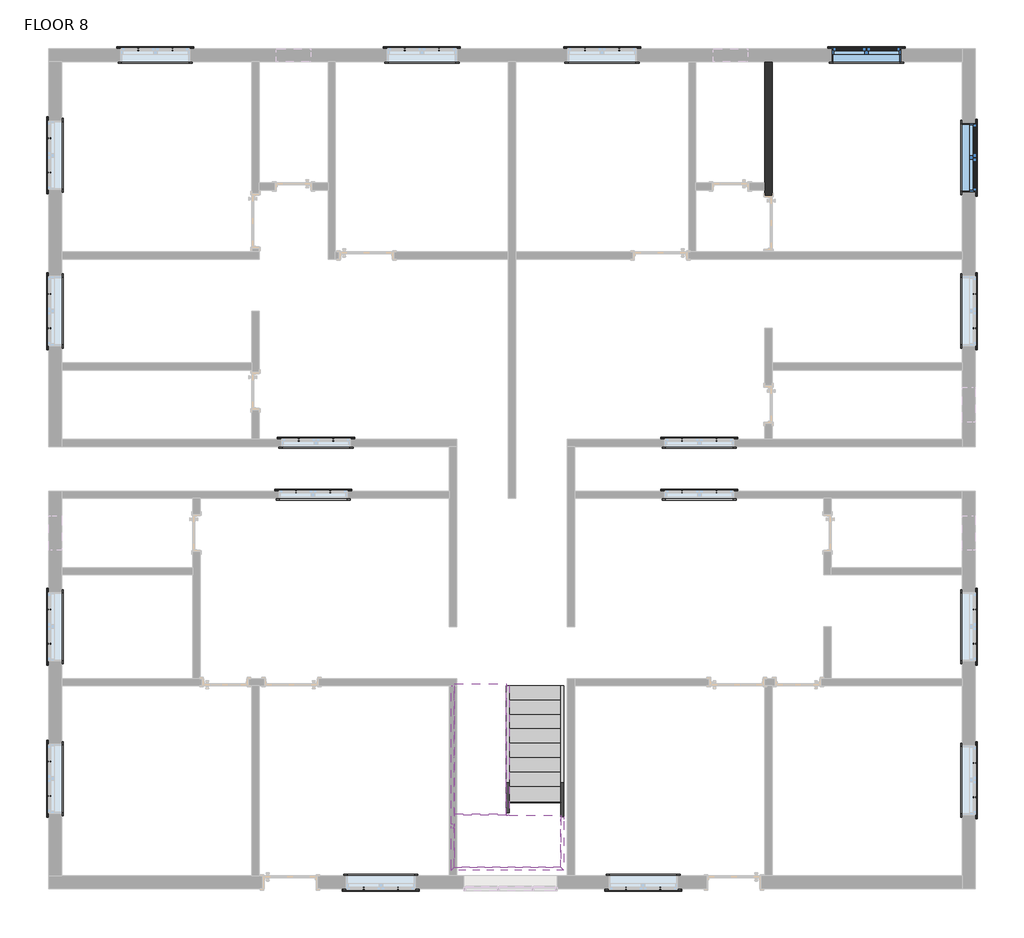
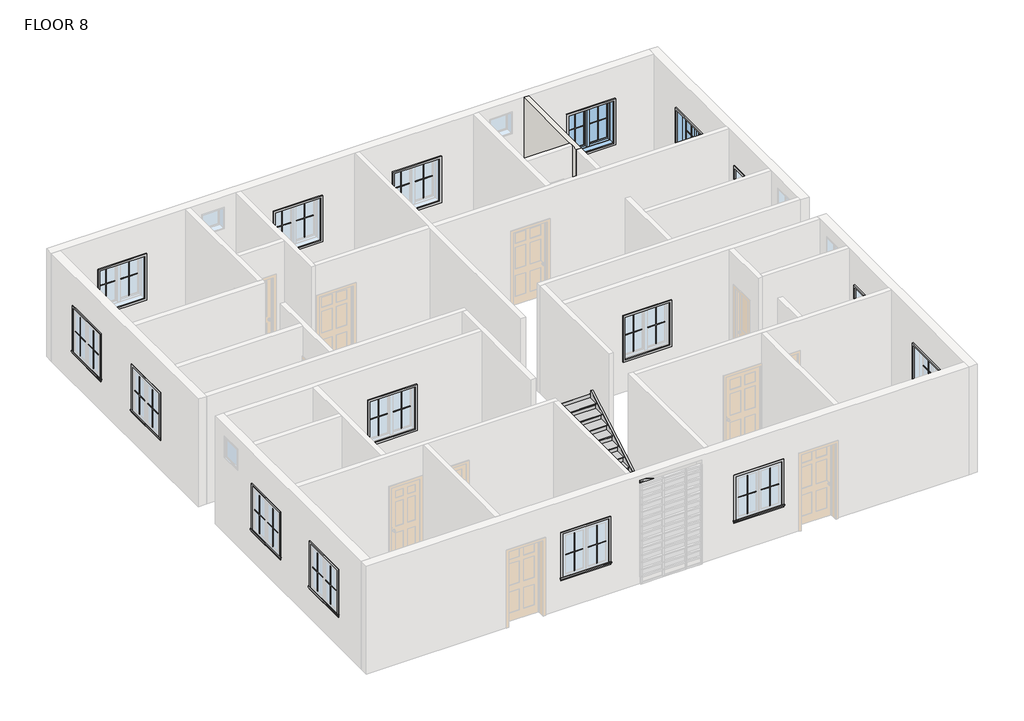
# One storey, part 4 of 4: 72 proxies, 7 members, 2 stair flights, 2 windows, 1 slab, 1 wall.
"""IFC4 building model written with IfcOpenShell, lengths in millimetres."""

from ifc_helpers import new_model, si_unit, frame, origin, place, context, project, spatial, polyline, outline, extrude, faceted_brep, transform, mapped, element, save
from components import muntin_pattern_2x2_muntin_pattern_2x2_4dfeb3f3, muntin_pattern_2x2_muntin_pattern_2x2_e852a7e4, trim_window_exterior_flat_with_sill_7cfdd449, trim_window_interior_flat_picture_frame_f1e0b15b, non_monolithic_landing_a6268fe4, stair_flight_98d8f9c6, stair_flight_dd50f657, window_9200f5ac

model = new_model("IFC4")

# Units and contexts
model_context = context("Model", 3, world=origin())
ifc_project = project(units=[si_unit("LENGTHUNIT", "METRE", prefix="MILLI")], contexts=[model_context])

# Site, building, storey
site = spatial("IfcSite", under=ifc_project)
building = spatial("IfcBuilding", under=site)
storey = spatial("IfcBuildingStorey", under=building, Name="FLOOR 8", Elevation=12744.7725604)

# Proxies
placement = place(None, origin())
muntin_pattern_2x2_muntin_pattern_2x2_shape = muntin_pattern_2x2_muntin_pattern_2x2_4dfeb3f3(model_context)
element("IfcBuildingElementProxy", 1, Name="Muntin Pattern_2x2 : Muntin Pattern_2x2", ObjectType="Muntin Pattern_2x2 : Muntin Pattern_2x2", at=placement, inside=storey, context=model_context, shape_type="MappedRepresentation", body=[
    mapped(muntin_pattern_2x2_muntin_pattern_2x2_shape, transform((-12420.8887331, 2059.7281164, 13729.0225604), x_axis=(0.0, 1.0, 0.0), y_axis=(-1.0, 0.0, 0.0), z_axis=(0.0, 0.0, 1.0))),
])
element("IfcBuildingElementProxy", 2, Name="Muntin Pattern_2x2 : Muntin Pattern_2x2", ObjectType="Muntin Pattern_2x2 : Muntin Pattern_2x2", at=placement, inside=storey, context=model_context, shape_type="MappedRepresentation", body=[
    mapped(muntin_pattern_2x2_muntin_pattern_2x2_shape, transform((-12420.8887331, 4803.7218664, 13729.0225604), x_axis=(0.0, 1.0, 0.0), y_axis=(-1.0, 0.0, 0.0), z_axis=(0.0, 0.0, 1.0))),
])
element("IfcBuildingElementProxy", 3, Name="Muntin Pattern_2x2 : Muntin Pattern_2x2", ObjectType="Muntin Pattern_2x2 : Muntin Pattern_2x2", at=placement, inside=storey, context=model_context, shape_type="MappedRepresentation", body=[
    mapped(muntin_pattern_2x2_muntin_pattern_2x2_shape, transform((-10854.0262331, 6977.8031164, 13729.0225604), x_axis=(1.0, 0.0, 0.0), y_axis=(0.0, 1.0, 0.0), z_axis=(0.0, 0.0, 1.0))),
])
element("IfcBuildingElementProxy", 4, Name="Muntin Pattern_2x2 : Muntin Pattern_2x2", ObjectType="Muntin Pattern_2x2 : Muntin Pattern_2x2", at=placement, inside=storey, context=model_context, shape_type="MappedRepresentation", body=[
    mapped(muntin_pattern_2x2_muntin_pattern_2x2_shape, transform((-6155.0262331, 6977.8031164, 13729.0225604), x_axis=(1.0, 0.0, 0.0), y_axis=(0.0, 1.0, 0.0), z_axis=(0.0, 0.0, 1.0))),
])
element("IfcBuildingElementProxy", 5, Name="Muntin Pattern_2x2 : Muntin Pattern_2x2", ObjectType="Muntin Pattern_2x2 : Muntin Pattern_2x2", at=placement, inside=storey, context=model_context, shape_type="MappedRepresentation", body=[
    mapped(muntin_pattern_2x2_muntin_pattern_2x2_shape, transform((-2980.0262331, 6977.8031164, 13729.0225604), x_axis=(1.0, 0.0, 0.0), y_axis=(0.0, 1.0, 0.0), z_axis=(0.0, 0.0, 1.0))),
])
element("IfcBuildingElementProxy", 6, Name="Muntin Pattern_2x2 : Muntin Pattern_2x2", ObjectType="Muntin Pattern_2x2 : Muntin Pattern_2x2", at=placement, inside=storey, context=model_context, shape_type="MappedRepresentation", body=[
    mapped(muntin_pattern_2x2_muntin_pattern_2x2_shape, transform((1680.8737669, 6977.8031164, 13729.0225604), x_axis=(1.0, 0.0, 0.0), y_axis=(0.0, 1.0, 0.0), z_axis=(0.0, 0.0, 1.0))),
])
element("IfcBuildingElementProxy", 7, Name="Muntin Pattern_2x2 : Muntin Pattern_2x2", ObjectType="Muntin Pattern_2x2 : Muntin Pattern_2x2", at=placement, inside=storey, context=model_context, shape_type="MappedRepresentation", body=[
    mapped(muntin_pattern_2x2_muntin_pattern_2x2_shape, transform((3892.2612669, 5371.2531164, 13729.0225604), x_axis=(0.0, -1.0, 0.0), y_axis=(1.0, 0.0, 0.0), z_axis=(0.0, 0.0, 1.0))),
])
element("IfcBuildingElementProxy", 8, Name="Muntin Pattern_2x2 : Muntin Pattern_2x2", ObjectType="Muntin Pattern_2x2 : Muntin Pattern_2x2", at=placement, inside=storey, context=model_context, shape_type="MappedRepresentation", body=[
    mapped(muntin_pattern_2x2_muntin_pattern_2x2_shape, transform((3892.2612669, 2666.1531164, 13729.0225604), x_axis=(0.0, -1.0, 0.0), y_axis=(1.0, 0.0, 0.0), z_axis=(0.0, 0.0, 1.0))),
])
element("IfcBuildingElementProxy", 9, Name="Muntin Pattern_2x2 : Muntin Pattern_2x2", ObjectType="Muntin Pattern_2x2 : Muntin Pattern_2x2", at=placement, inside=storey, context=model_context, shape_type="MappedRepresentation", body=[
    mapped(muntin_pattern_2x2_muntin_pattern_2x2_shape, transform((3892.2612669, -2896.4468836, 13729.0225604), x_axis=(0.0, -1.0, 0.0), y_axis=(1.0, 0.0, 0.0), z_axis=(0.0, 0.0, 1.0))),
])
element("IfcBuildingElementProxy", 10, Name="Muntin Pattern_2x2 : Muntin Pattern_2x2", ObjectType="Muntin Pattern_2x2 : Muntin Pattern_2x2", at=placement, inside=storey, context=model_context, shape_type="MappedRepresentation", body=[
    mapped(muntin_pattern_2x2_muntin_pattern_2x2_shape, transform((3892.2612669, -5601.5468836, 13729.0225604), x_axis=(0.0, -1.0, 0.0), y_axis=(1.0, 0.0, 0.0), z_axis=(0.0, 0.0, 1.0))),
])
element("IfcBuildingElementProxy", 11, Name="Muntin Pattern_2x2 : Muntin Pattern_2x2", ObjectType="Muntin Pattern_2x2 : Muntin Pattern_2x2", at=placement, inside=storey, context=model_context, shape_type="MappedRepresentation", body=[
    mapped(muntin_pattern_2x2_muntin_pattern_2x2_shape, transform((-1649.7012331, -7812.9343836, 13729.0225604), x_axis=(-1.0, 0.0, 0.0), y_axis=(0.0, -1.0, 0.0), z_axis=(0.0, 0.0, 1.0))),
])
element("IfcBuildingElementProxy", 12, Name="Muntin Pattern_2x2 : Muntin Pattern_2x2", ObjectType="Muntin Pattern_2x2 : Muntin Pattern_2x2", at=placement, inside=storey, context=model_context, shape_type="MappedRepresentation", body=[
    mapped(muntin_pattern_2x2_muntin_pattern_2x2_shape, transform((-6272.5012331, -7812.9343836, 13729.0225604), x_axis=(-1.0, 0.0, 0.0), y_axis=(0.0, -1.0, 0.0), z_axis=(0.0, 0.0, 1.0))),
])
element("IfcBuildingElementProxy", 13, Name="Muntin Pattern_2x2 : Muntin Pattern_2x2", ObjectType="Muntin Pattern_2x2 : Muntin Pattern_2x2", at=placement, inside=storey, context=model_context, shape_type="MappedRepresentation", body=[
    mapped(muntin_pattern_2x2_muntin_pattern_2x2_shape, transform((-12420.8887331, -6182.5718836, 13729.0225604), x_axis=(0.0, 1.0, 0.0), y_axis=(-1.0, 0.0, 0.0), z_axis=(0.0, 0.0, 1.0))),
])
element("IfcBuildingElementProxy", 14, Name="Muntin Pattern_2x2 : Muntin Pattern_2x2", ObjectType="Muntin Pattern_2x2 : Muntin Pattern_2x2", at=placement, inside=storey, context=model_context, shape_type="MappedRepresentation", body=[
    mapped(muntin_pattern_2x2_muntin_pattern_2x2_shape, transform((-12420.8887331, -3502.8718836, 13729.0225604), x_axis=(0.0, 1.0, 0.0), y_axis=(-1.0, 0.0, 0.0), z_axis=(0.0, 0.0, 1.0))),
])
element("IfcBuildingElementProxy", 15, Name="Muntin Pattern_2x2 : Muntin Pattern_2x2", ObjectType="Muntin Pattern_2x2 : Muntin Pattern_2x2", at=placement, inside=storey, context=model_context, shape_type="MappedRepresentation", body=[
    mapped(muntin_pattern_2x2_muntin_pattern_2x2_shape, transform((-8072.7262331, -821.5843836, 13729.0225604), x_axis=(1.0, 0.0, 0.0), y_axis=(0.0, 1.0, 0.0), z_axis=(0.0, 0.0, 1.0))),
])
element("IfcBuildingElementProxy", 16, Name="Muntin Pattern_2x2 : Muntin Pattern_2x2", ObjectType="Muntin Pattern_2x2 : Muntin Pattern_2x2", at=placement, inside=storey, context=model_context, shape_type="MappedRepresentation", body=[
    mapped(muntin_pattern_2x2_muntin_pattern_2x2_shape, transform((-8021.9262331, 92.8156164, 13729.0225604), x_axis=(1.0, 0.0, 0.0), y_axis=(0.0, 1.0, 0.0), z_axis=(0.0, 0.0, 1.0))),
])
element("IfcBuildingElementProxy", 17, Name="Muntin Pattern_2x2 : Muntin Pattern_2x2", ObjectType="Muntin Pattern_2x2 : Muntin Pattern_2x2", at=placement, inside=storey, context=model_context, shape_type="MappedRepresentation", body=[
    mapped(muntin_pattern_2x2_muntin_pattern_2x2_shape, transform((-1265.5262331, -821.5843836, 13729.0225604), x_axis=(1.0, 0.0, 0.0), y_axis=(0.0, 1.0, 0.0), z_axis=(0.0, 0.0, 1.0))),
])
element("IfcBuildingElementProxy", 18, Name="Muntin Pattern_2x2 : Muntin Pattern_2x2", ObjectType="Muntin Pattern_2x2 : Muntin Pattern_2x2", at=placement, inside=storey, context=model_context, shape_type="MappedRepresentation", body=[
    mapped(muntin_pattern_2x2_muntin_pattern_2x2_shape, transform((-1265.5262331, 92.8156164, 13729.0225604), x_axis=(1.0, 0.0, 0.0), y_axis=(0.0, 1.0, 0.0), z_axis=(0.0, 0.0, 1.0))),
])
muntin_pattern_2x2_muntin_pattern_2x2_2_shape = muntin_pattern_2x2_muntin_pattern_2x2_e852a7e4(model_context)
element("IfcBuildingElementProxy", 19, Name="Muntin Pattern_2x2 : Muntin Pattern_2x2", ObjectType="Muntin Pattern_2x2 : Muntin Pattern_2x2", at=placement, inside=storey, context=model_context, shape_type="MappedRepresentation", body=[
    mapped(muntin_pattern_2x2_muntin_pattern_2x2_2_shape, transform((-12420.8887331, 2666.1531164, 13729.0225604), x_axis=(0.0, -1.0, 0.0), y_axis=(1.0, 0.0, 0.0), z_axis=(0.0, 0.0, 1.0))),
])
element("IfcBuildingElementProxy", 20, Name="Muntin Pattern_2x2 : Muntin Pattern_2x2", ObjectType="Muntin Pattern_2x2 : Muntin Pattern_2x2", at=placement, inside=storey, context=model_context, shape_type="MappedRepresentation", body=[
    mapped(muntin_pattern_2x2_muntin_pattern_2x2_2_shape, transform((-12420.8887331, 5410.1468664, 13729.0225604), x_axis=(0.0, -1.0, 0.0), y_axis=(1.0, 0.0, 0.0), z_axis=(0.0, 0.0, 1.0))),
])
element("IfcBuildingElementProxy", 21, Name="Muntin Pattern_2x2 : Muntin Pattern_2x2", ObjectType="Muntin Pattern_2x2 : Muntin Pattern_2x2", at=placement, inside=storey, context=model_context, shape_type="MappedRepresentation", body=[
    mapped(muntin_pattern_2x2_muntin_pattern_2x2_2_shape, transform((-10247.6012331, 6977.8031164, 13729.0225604), x_axis=(-1.0, 0.0, 0.0), y_axis=(0.0, -1.0, 0.0), z_axis=(0.0, 0.0, 1.0))),
])
element("IfcBuildingElementProxy", 22, Name="Muntin Pattern_2x2 : Muntin Pattern_2x2", ObjectType="Muntin Pattern_2x2 : Muntin Pattern_2x2", at=placement, inside=storey, context=model_context, shape_type="MappedRepresentation", body=[
    mapped(muntin_pattern_2x2_muntin_pattern_2x2_2_shape, transform((-5548.6012331, 6977.8031164, 13729.0225604), x_axis=(-1.0, 0.0, 0.0), y_axis=(0.0, -1.0, 0.0), z_axis=(0.0, 0.0, 1.0))),
])
element("IfcBuildingElementProxy", 23, Name="Muntin Pattern_2x2 : Muntin Pattern_2x2", ObjectType="Muntin Pattern_2x2 : Muntin Pattern_2x2", at=placement, inside=storey, context=model_context, shape_type="MappedRepresentation", body=[
    mapped(muntin_pattern_2x2_muntin_pattern_2x2_2_shape, transform((-2373.6012331, 6977.8031164, 13729.0225604), x_axis=(-1.0, 0.0, 0.0), y_axis=(0.0, -1.0, 0.0), z_axis=(0.0, 0.0, 1.0))),
])
element("IfcBuildingElementProxy", 24, Name="Muntin Pattern_2x2 : Muntin Pattern_2x2", ObjectType="Muntin Pattern_2x2 : Muntin Pattern_2x2", at=placement, inside=storey, context=model_context, shape_type="MappedRepresentation", body=[
    mapped(muntin_pattern_2x2_muntin_pattern_2x2_2_shape, transform((2287.2987669, 6977.8031164, 13729.0225604), x_axis=(-1.0, 0.0, 0.0), y_axis=(0.0, -1.0, 0.0), z_axis=(0.0, 0.0, 1.0))),
])
element("IfcBuildingElementProxy", 25, Name="Muntin Pattern_2x2 : Muntin Pattern_2x2", ObjectType="Muntin Pattern_2x2 : Muntin Pattern_2x2", at=placement, inside=storey, context=model_context, shape_type="MappedRepresentation", body=[
    mapped(muntin_pattern_2x2_muntin_pattern_2x2_2_shape, transform((3892.2612669, 4764.8281164, 13729.0225604), x_axis=(0.0, 1.0, 0.0), y_axis=(-1.0, 0.0, 0.0), z_axis=(0.0, 0.0, 1.0))),
])
element("IfcBuildingElementProxy", 26, Name="Muntin Pattern_2x2 : Muntin Pattern_2x2", ObjectType="Muntin Pattern_2x2 : Muntin Pattern_2x2", at=placement, inside=storey, context=model_context, shape_type="MappedRepresentation", body=[
    mapped(muntin_pattern_2x2_muntin_pattern_2x2_2_shape, transform((3892.2612669, 2059.7281164, 13729.0225604), x_axis=(0.0, 1.0, 0.0), y_axis=(-1.0, 0.0, 0.0), z_axis=(0.0, 0.0, 1.0))),
])
element("IfcBuildingElementProxy", 27, Name="Muntin Pattern_2x2 : Muntin Pattern_2x2", ObjectType="Muntin Pattern_2x2 : Muntin Pattern_2x2", at=placement, inside=storey, context=model_context, shape_type="MappedRepresentation", body=[
    mapped(muntin_pattern_2x2_muntin_pattern_2x2_2_shape, transform((3892.2612669, -3502.8718836, 13729.0225604), x_axis=(0.0, 1.0, 0.0), y_axis=(-1.0, 0.0, 0.0), z_axis=(0.0, 0.0, 1.0))),
])
element("IfcBuildingElementProxy", 28, Name="Muntin Pattern_2x2 : Muntin Pattern_2x2", ObjectType="Muntin Pattern_2x2 : Muntin Pattern_2x2", at=placement, inside=storey, context=model_context, shape_type="MappedRepresentation", body=[
    mapped(muntin_pattern_2x2_muntin_pattern_2x2_2_shape, transform((3892.2612669, -6207.9718836, 13729.0225604), x_axis=(0.0, 1.0, 0.0), y_axis=(-1.0, 0.0, 0.0), z_axis=(0.0, 0.0, 1.0))),
])
element("IfcBuildingElementProxy", 29, Name="Muntin Pattern_2x2 : Muntin Pattern_2x2", ObjectType="Muntin Pattern_2x2 : Muntin Pattern_2x2", at=placement, inside=storey, context=model_context, shape_type="MappedRepresentation", body=[
    mapped(muntin_pattern_2x2_muntin_pattern_2x2_2_shape, transform((-2256.1262331, -7812.9343836, 13729.0225604), x_axis=(1.0, 0.0, 0.0), y_axis=(0.0, 1.0, 0.0), z_axis=(0.0, 0.0, 1.0))),
])
element("IfcBuildingElementProxy", 30, Name="Muntin Pattern_2x2 : Muntin Pattern_2x2", ObjectType="Muntin Pattern_2x2 : Muntin Pattern_2x2", at=placement, inside=storey, context=model_context, shape_type="MappedRepresentation", body=[
    mapped(muntin_pattern_2x2_muntin_pattern_2x2_2_shape, transform((-6878.9262331, -7812.9343836, 13729.0225604), x_axis=(1.0, 0.0, 0.0), y_axis=(0.0, 1.0, 0.0), z_axis=(0.0, 0.0, 1.0))),
])
element("IfcBuildingElementProxy", 31, Name="Muntin Pattern_2x2 : Muntin Pattern_2x2", ObjectType="Muntin Pattern_2x2 : Muntin Pattern_2x2", at=placement, inside=storey, context=model_context, shape_type="MappedRepresentation", body=[
    mapped(muntin_pattern_2x2_muntin_pattern_2x2_2_shape, transform((-12420.8887331, -5576.1468836, 13729.0225604), x_axis=(0.0, -1.0, 0.0), y_axis=(1.0, 0.0, 0.0), z_axis=(0.0, 0.0, 1.0))),
])
element("IfcBuildingElementProxy", 32, Name="Muntin Pattern_2x2 : Muntin Pattern_2x2", ObjectType="Muntin Pattern_2x2 : Muntin Pattern_2x2", at=placement, inside=storey, context=model_context, shape_type="MappedRepresentation", body=[
    mapped(muntin_pattern_2x2_muntin_pattern_2x2_2_shape, transform((-12420.8887331, -2896.4468836, 13729.0225604), x_axis=(0.0, -1.0, 0.0), y_axis=(1.0, 0.0, 0.0), z_axis=(0.0, 0.0, 1.0))),
])
element("IfcBuildingElementProxy", 33, Name="Muntin Pattern_2x2 : Muntin Pattern_2x2", ObjectType="Muntin Pattern_2x2 : Muntin Pattern_2x2", at=placement, inside=storey, context=model_context, shape_type="MappedRepresentation", body=[
    mapped(muntin_pattern_2x2_muntin_pattern_2x2_2_shape, transform((-7466.3012331, -821.5843836, 13729.0225604), x_axis=(-1.0, 0.0, 0.0), y_axis=(0.0, -1.0, 0.0), z_axis=(0.0, 0.0, 1.0))),
])
element("IfcBuildingElementProxy", 34, Name="Muntin Pattern_2x2 : Muntin Pattern_2x2", ObjectType="Muntin Pattern_2x2 : Muntin Pattern_2x2", at=placement, inside=storey, context=model_context, shape_type="MappedRepresentation", body=[
    mapped(muntin_pattern_2x2_muntin_pattern_2x2_2_shape, transform((-7415.5012331, 92.8156164, 13729.0225604), x_axis=(-1.0, 0.0, 0.0), y_axis=(0.0, -1.0, 0.0), z_axis=(0.0, 0.0, 1.0))),
])
element("IfcBuildingElementProxy", 35, Name="Muntin Pattern_2x2 : Muntin Pattern_2x2", ObjectType="Muntin Pattern_2x2 : Muntin Pattern_2x2", at=placement, inside=storey, context=model_context, shape_type="MappedRepresentation", body=[
    mapped(muntin_pattern_2x2_muntin_pattern_2x2_2_shape, transform((-659.1012331, -821.5843836, 13729.0225604), x_axis=(-1.0, 0.0, 0.0), y_axis=(0.0, -1.0, 0.0), z_axis=(0.0, 0.0, 1.0))),
])
element("IfcBuildingElementProxy", 36, Name="Muntin Pattern_2x2 : Muntin Pattern_2x2", ObjectType="Muntin Pattern_2x2 : Muntin Pattern_2x2", at=placement, inside=storey, context=model_context, shape_type="MappedRepresentation", body=[
    mapped(muntin_pattern_2x2_muntin_pattern_2x2_2_shape, transform((-659.1012331, 92.8156164, 13729.0225604), x_axis=(-1.0, 0.0, 0.0), y_axis=(0.0, -1.0, 0.0), z_axis=(0.0, 0.0, 1.0))),
])
trim_window_exterior_flat_with_sill_shape = trim_window_exterior_flat_with_sill_7cfdd449(model_context)
element("IfcBuildingElementProxy", 37, Name="Trim-Window-Exterior-Flat : with Sill", ObjectType="Trim-Window-Exterior-Flat : with Sill", at=placement, inside=storey, context=model_context, shape_type="MappedRepresentation", body=[
    mapped(trim_window_exterior_flat_with_sill_shape, transform((-12430.4137331, 2362.9406164, 14878.3725604), x_axis=(0.0, -1.0, 0.0), y_axis=(0.0, 0.0, 1.0), z_axis=(-1.0, 0.0, 0.0))),
])
element("IfcBuildingElementProxy", 38, Name="Trim-Window-Exterior-Flat : with Sill", ObjectType="Trim-Window-Exterior-Flat : with Sill", at=placement, inside=storey, context=model_context, shape_type="MappedRepresentation", body=[
    mapped(trim_window_exterior_flat_with_sill_shape, transform((-12430.4137331, 5106.9343664, 14878.3725604), x_axis=(0.0, -1.0, 0.0), y_axis=(0.0, 0.0, 1.0), z_axis=(-1.0, 0.0, 0.0))),
])
element("IfcBuildingElementProxy", 39, Name="Trim-Window-Exterior-Flat : with Sill", ObjectType="Trim-Window-Exterior-Flat : with Sill", at=placement, inside=storey, context=model_context, shape_type="MappedRepresentation", body=[
    mapped(trim_window_exterior_flat_with_sill_shape, transform((-10550.8137331, 6987.3281164, 14878.3725604), x_axis=(-1.0, 0.0, 0.0), y_axis=(0.0, 0.0, 1.0), z_axis=(0.0, 1.0, 0.0))),
])
element("IfcBuildingElementProxy", 40, Name="Trim-Window-Exterior-Flat : with Sill", ObjectType="Trim-Window-Exterior-Flat : with Sill", at=placement, inside=storey, context=model_context, shape_type="MappedRepresentation", body=[
    mapped(trim_window_exterior_flat_with_sill_shape, transform((-5851.8137331, 6987.3281164, 14878.3725604), x_axis=(-1.0, 0.0, 0.0), y_axis=(0.0, 0.0, 1.0), z_axis=(0.0, 1.0, 0.0))),
])
element("IfcBuildingElementProxy", 41, Name="Trim-Window-Exterior-Flat : with Sill", ObjectType="Trim-Window-Exterior-Flat : with Sill", at=placement, inside=storey, context=model_context, shape_type="MappedRepresentation", body=[
    mapped(trim_window_exterior_flat_with_sill_shape, transform((-2676.8137331, 6987.3281164, 14878.3725604), x_axis=(-1.0, 0.0, 0.0), y_axis=(0.0, 0.0, 1.0), z_axis=(0.0, 1.0, 0.0))),
])
element("IfcBuildingElementProxy", 42, Name="Trim-Window-Exterior-Flat : with Sill", ObjectType="Trim-Window-Exterior-Flat : with Sill", at=placement, inside=storey, context=model_context, shape_type="MappedRepresentation", body=[
    mapped(trim_window_exterior_flat_with_sill_shape, transform((1984.0862669, 6987.3281164, 14878.3725604), x_axis=(-1.0, 0.0, 0.0), y_axis=(0.0, 0.0, 1.0), z_axis=(0.0, 1.0, 0.0))),
])
element("IfcBuildingElementProxy", 43, Name="Trim-Window-Exterior-Flat : with Sill", ObjectType="Trim-Window-Exterior-Flat : with Sill", at=placement, inside=storey, context=model_context, shape_type="MappedRepresentation", body=[
    mapped(trim_window_exterior_flat_with_sill_shape, transform((3901.7862669, 5068.0406164, 14878.3725604), x_axis=(0.0, 1.0, 0.0), y_axis=(0.0, 0.0, 1.0), z_axis=(1.0, 0.0, 0.0))),
])
element("IfcBuildingElementProxy", 44, Name="Trim-Window-Exterior-Flat : with Sill", ObjectType="Trim-Window-Exterior-Flat : with Sill", at=placement, inside=storey, context=model_context, shape_type="MappedRepresentation", body=[
    mapped(trim_window_exterior_flat_with_sill_shape, transform((3901.7862669, 2362.9406164, 14878.3725604), x_axis=(0.0, 1.0, 0.0), y_axis=(0.0, 0.0, 1.0), z_axis=(1.0, 0.0, 0.0))),
])
element("IfcBuildingElementProxy", 45, Name="Trim-Window-Exterior-Flat : with Sill", ObjectType="Trim-Window-Exterior-Flat : with Sill", at=placement, inside=storey, context=model_context, shape_type="MappedRepresentation", body=[
    mapped(trim_window_exterior_flat_with_sill_shape, transform((3901.7862669, -3199.6593836, 14878.3725604), x_axis=(0.0, 1.0, 0.0), y_axis=(0.0, 0.0, 1.0), z_axis=(1.0, 0.0, 0.0))),
])
element("IfcBuildingElementProxy", 46, Name="Trim-Window-Exterior-Flat : with Sill", ObjectType="Trim-Window-Exterior-Flat : with Sill", at=placement, inside=storey, context=model_context, shape_type="MappedRepresentation", body=[
    mapped(trim_window_exterior_flat_with_sill_shape, transform((3901.7862669, -5904.7593836, 14878.3725604), x_axis=(0.0, 1.0, 0.0), y_axis=(0.0, 0.0, 1.0), z_axis=(1.0, 0.0, 0.0))),
])
element("IfcBuildingElementProxy", 47, Name="Trim-Window-Exterior-Flat : with Sill", ObjectType="Trim-Window-Exterior-Flat : with Sill", at=placement, inside=storey, context=model_context, shape_type="MappedRepresentation", body=[
    mapped(trim_window_exterior_flat_with_sill_shape, transform((-1952.9137331, -7822.4593836, 14878.3725604), x_axis=(1.0, 0.0, 0.0), y_axis=(0.0, 0.0, 1.0), z_axis=(0.0, -1.0, 0.0))),
])
element("IfcBuildingElementProxy", 48, Name="Trim-Window-Exterior-Flat : with Sill", ObjectType="Trim-Window-Exterior-Flat : with Sill", at=placement, inside=storey, context=model_context, shape_type="MappedRepresentation", body=[
    mapped(trim_window_exterior_flat_with_sill_shape, transform((-6575.7137331, -7822.4593836, 14878.3725604), x_axis=(1.0, 0.0, 0.0), y_axis=(0.0, 0.0, 1.0), z_axis=(0.0, -1.0, 0.0))),
])
element("IfcBuildingElementProxy", 49, Name="Trim-Window-Exterior-Flat : with Sill", ObjectType="Trim-Window-Exterior-Flat : with Sill", at=placement, inside=storey, context=model_context, shape_type="MappedRepresentation", body=[
    mapped(trim_window_exterior_flat_with_sill_shape, transform((-12430.4137331, -5879.3593836, 14878.3725604), x_axis=(0.0, -1.0, 0.0), y_axis=(0.0, 0.0, 1.0), z_axis=(-1.0, 0.0, 0.0))),
])
element("IfcBuildingElementProxy", 50, Name="Trim-Window-Exterior-Flat : with Sill", ObjectType="Trim-Window-Exterior-Flat : with Sill", at=placement, inside=storey, context=model_context, shape_type="MappedRepresentation", body=[
    mapped(trim_window_exterior_flat_with_sill_shape, transform((-12430.4137331, -3199.6593836, 14878.3725604), x_axis=(0.0, -1.0, 0.0), y_axis=(0.0, 0.0, 1.0), z_axis=(-1.0, 0.0, 0.0))),
])
element("IfcBuildingElementProxy", 51, Name="Trim-Window-Exterior-Flat : with Sill", ObjectType="Trim-Window-Exterior-Flat : with Sill", at=placement, inside=storey, context=model_context, shape_type="MappedRepresentation", body=[
    mapped(trim_window_exterior_flat_with_sill_shape, transform((-7769.5137331, -812.0593836, 14878.3725604), x_axis=(-1.0, 0.0, 0.0), y_axis=(0.0, 0.0, 1.0), z_axis=(0.0, 1.0, 0.0))),
])
element("IfcBuildingElementProxy", 52, Name="Trim-Window-Exterior-Flat : with Sill", ObjectType="Trim-Window-Exterior-Flat : with Sill", at=placement, inside=storey, context=model_context, shape_type="MappedRepresentation", body=[
    mapped(trim_window_exterior_flat_with_sill_shape, transform((-7718.7137331, 102.3406164, 14878.3725604), x_axis=(-1.0, 0.0, 0.0), y_axis=(0.0, 0.0, 1.0), z_axis=(0.0, 1.0, 0.0))),
])
element("IfcBuildingElementProxy", 53, Name="Trim-Window-Exterior-Flat : with Sill", ObjectType="Trim-Window-Exterior-Flat : with Sill", at=placement, inside=storey, context=model_context, shape_type="MappedRepresentation", body=[
    mapped(trim_window_exterior_flat_with_sill_shape, transform((-962.3137331, -812.0593836, 14878.3725604), x_axis=(-1.0, 0.0, 0.0), y_axis=(0.0, 0.0, 1.0), z_axis=(0.0, 1.0, 0.0))),
])
element("IfcBuildingElementProxy", 54, Name="Trim-Window-Exterior-Flat : with Sill", ObjectType="Trim-Window-Exterior-Flat : with Sill", at=placement, inside=storey, context=model_context, shape_type="MappedRepresentation", body=[
    mapped(trim_window_exterior_flat_with_sill_shape, transform((-962.3137331, 102.3406164, 14878.3725604), x_axis=(-1.0, 0.0, 0.0), y_axis=(0.0, 0.0, 1.0), z_axis=(0.0, 1.0, 0.0))),
])
trim_window_interior_flat_picture_frame_shape = trim_window_interior_flat_picture_frame_f1e0b15b(model_context)
element("IfcBuildingElementProxy", 55, Name="Trim-Window-Interior-Flat : Picture Frame", ObjectType="Trim-Window-Interior-Flat : Picture Frame", at=placement, inside=storey, context=model_context, shape_type="MappedRepresentation", body=[
    mapped(trim_window_interior_flat_picture_frame_shape, transform((-12201.8137331, 2362.9406164, 14878.3725604), x_axis=(0.0, 1.0, 0.0), y_axis=(0.0, 0.0, 1.0), z_axis=(1.0, 0.0, 0.0))),
])
element("IfcBuildingElementProxy", 56, Name="Trim-Window-Interior-Flat : Picture Frame", ObjectType="Trim-Window-Interior-Flat : Picture Frame", at=placement, inside=storey, context=model_context, shape_type="MappedRepresentation", body=[
    mapped(trim_window_interior_flat_picture_frame_shape, transform((-12201.8137331, 5106.9343664, 14878.3725604), x_axis=(0.0, 1.0, 0.0), y_axis=(0.0, 0.0, 1.0), z_axis=(1.0, 0.0, 0.0))),
])
element("IfcBuildingElementProxy", 57, Name="Trim-Window-Interior-Flat : Picture Frame", ObjectType="Trim-Window-Interior-Flat : Picture Frame", at=placement, inside=storey, context=model_context, shape_type="MappedRepresentation", body=[
    mapped(trim_window_interior_flat_picture_frame_shape, transform((-10550.8137331, 6758.7281164, 14878.3725604), x_axis=(1.0, 0.0, 0.0), y_axis=(0.0, 0.0, 1.0), z_axis=(0.0, -1.0, 0.0))),
])
element("IfcBuildingElementProxy", 58, Name="Trim-Window-Interior-Flat : Picture Frame", ObjectType="Trim-Window-Interior-Flat : Picture Frame", at=placement, inside=storey, context=model_context, shape_type="MappedRepresentation", body=[
    mapped(trim_window_interior_flat_picture_frame_shape, transform((-5851.8137331, 6758.7281164, 14878.3725604), x_axis=(1.0, 0.0, 0.0), y_axis=(0.0, 0.0, 1.0), z_axis=(0.0, -1.0, 0.0))),
])
element("IfcBuildingElementProxy", 59, Name="Trim-Window-Interior-Flat : Picture Frame", ObjectType="Trim-Window-Interior-Flat : Picture Frame", at=placement, inside=storey, context=model_context, shape_type="MappedRepresentation", body=[
    mapped(trim_window_interior_flat_picture_frame_shape, transform((-2676.8137331, 6758.7281164, 14878.3725604), x_axis=(1.0, 0.0, 0.0), y_axis=(0.0, 0.0, 1.0), z_axis=(0.0, -1.0, 0.0))),
])
element("IfcBuildingElementProxy", 60, Name="Trim-Window-Interior-Flat : Picture Frame", ObjectType="Trim-Window-Interior-Flat : Picture Frame", at=placement, inside=storey, context=model_context, shape_type="MappedRepresentation", body=[
    mapped(trim_window_interior_flat_picture_frame_shape, transform((1984.0862669, 6758.7281164, 14878.3725604), x_axis=(1.0, 0.0, 0.0), y_axis=(0.0, 0.0, 1.0), z_axis=(0.0, -1.0, 0.0))),
])
element("IfcBuildingElementProxy", 61, Name="Trim-Window-Interior-Flat : Picture Frame", ObjectType="Trim-Window-Interior-Flat : Picture Frame", at=placement, inside=storey, context=model_context, shape_type="MappedRepresentation", body=[
    mapped(trim_window_interior_flat_picture_frame_shape, transform((3673.1862669, 5068.0406164, 14878.3725604), x_axis=(0.0, -1.0, 0.0), y_axis=(0.0, 0.0, 1.0), z_axis=(-1.0, 0.0, 0.0))),
])
element("IfcBuildingElementProxy", 62, Name="Trim-Window-Interior-Flat : Picture Frame", ObjectType="Trim-Window-Interior-Flat : Picture Frame", at=placement, inside=storey, context=model_context, shape_type="MappedRepresentation", body=[
    mapped(trim_window_interior_flat_picture_frame_shape, transform((3673.1862669, 2362.9406164, 14878.3725604), x_axis=(0.0, -1.0, 0.0), y_axis=(0.0, 0.0, 1.0), z_axis=(-1.0, 0.0, 0.0))),
])
element("IfcBuildingElementProxy", 63, Name="Trim-Window-Interior-Flat : Picture Frame", ObjectType="Trim-Window-Interior-Flat : Picture Frame", at=placement, inside=storey, context=model_context, shape_type="MappedRepresentation", body=[
    mapped(trim_window_interior_flat_picture_frame_shape, transform((3673.1862669, -3199.6593836, 14878.3725604), x_axis=(0.0, -1.0, 0.0), y_axis=(0.0, 0.0, 1.0), z_axis=(-1.0, 0.0, 0.0))),
])
element("IfcBuildingElementProxy", 64, Name="Trim-Window-Interior-Flat : Picture Frame", ObjectType="Trim-Window-Interior-Flat : Picture Frame", at=placement, inside=storey, context=model_context, shape_type="MappedRepresentation", body=[
    mapped(trim_window_interior_flat_picture_frame_shape, transform((3673.1862669, -5904.7593836, 14878.3725604), x_axis=(0.0, -1.0, 0.0), y_axis=(0.0, 0.0, 1.0), z_axis=(-1.0, 0.0, 0.0))),
])
element("IfcBuildingElementProxy", 65, Name="Trim-Window-Interior-Flat : Picture Frame", ObjectType="Trim-Window-Interior-Flat : Picture Frame", at=placement, inside=storey, context=model_context, shape_type="MappedRepresentation", body=[
    mapped(trim_window_interior_flat_picture_frame_shape, transform((-1952.9137331, -7593.8593836, 14878.3725604), x_axis=(-1.0, 0.0, 0.0), y_axis=(0.0, 0.0, 1.0), z_axis=(0.0, 1.0, 0.0))),
])
element("IfcBuildingElementProxy", 66, Name="Trim-Window-Interior-Flat : Picture Frame", ObjectType="Trim-Window-Interior-Flat : Picture Frame", at=placement, inside=storey, context=model_context, shape_type="MappedRepresentation", body=[
    mapped(trim_window_interior_flat_picture_frame_shape, transform((-6575.7137331, -7593.8593836, 14878.3725604), x_axis=(-1.0, 0.0, 0.0), y_axis=(0.0, 0.0, 1.0), z_axis=(0.0, 1.0, 0.0))),
])
element("IfcBuildingElementProxy", 67, Name="Trim-Window-Interior-Flat : Picture Frame", ObjectType="Trim-Window-Interior-Flat : Picture Frame", at=placement, inside=storey, context=model_context, shape_type="MappedRepresentation", body=[
    mapped(trim_window_interior_flat_picture_frame_shape, transform((-12201.8137331, -5879.3593836, 14878.3725604), x_axis=(0.0, 1.0, 0.0), y_axis=(0.0, 0.0, 1.0), z_axis=(1.0, 0.0, 0.0))),
])
element("IfcBuildingElementProxy", 68, Name="Trim-Window-Interior-Flat : Picture Frame", ObjectType="Trim-Window-Interior-Flat : Picture Frame", at=placement, inside=storey, context=model_context, shape_type="MappedRepresentation", body=[
    mapped(trim_window_interior_flat_picture_frame_shape, transform((-12201.8137331, -3199.6593836, 14878.3725604), x_axis=(0.0, 1.0, 0.0), y_axis=(0.0, 0.0, 1.0), z_axis=(1.0, 0.0, 0.0))),
])
element("IfcBuildingElementProxy", 69, Name="Trim-Window-Interior-Flat : Picture Frame", ObjectType="Trim-Window-Interior-Flat : Picture Frame", at=placement, inside=storey, context=model_context, shape_type="MappedRepresentation", body=[
    mapped(trim_window_interior_flat_picture_frame_shape, transform((-7769.5137331, -939.0593836, 14878.3725604), x_axis=(1.0, 0.0, 0.0), y_axis=(0.0, 0.0, 1.0), z_axis=(0.0, -1.0, 0.0))),
])
element("IfcBuildingElementProxy", 70, Name="Trim-Window-Interior-Flat : Picture Frame", ObjectType="Trim-Window-Interior-Flat : Picture Frame", at=placement, inside=storey, context=model_context, shape_type="MappedRepresentation", body=[
    mapped(trim_window_interior_flat_picture_frame_shape, transform((-7718.7137331, -24.6593836, 14878.3725604), x_axis=(1.0, 0.0, 0.0), y_axis=(0.0, 0.0, 1.0), z_axis=(0.0, -1.0, 0.0))),
])
element("IfcBuildingElementProxy", 71, Name="Trim-Window-Interior-Flat : Picture Frame", ObjectType="Trim-Window-Interior-Flat : Picture Frame", at=placement, inside=storey, context=model_context, shape_type="MappedRepresentation", body=[
    mapped(trim_window_interior_flat_picture_frame_shape, transform((-962.3137331, -939.0593836, 14878.3725604), x_axis=(1.0, 0.0, 0.0), y_axis=(0.0, 0.0, 1.0), z_axis=(0.0, -1.0, 0.0))),
])
element("IfcBuildingElementProxy", 72, Name="Trim-Window-Interior-Flat : Picture Frame", ObjectType="Trim-Window-Interior-Flat : Picture Frame", at=placement, inside=storey, context=model_context, shape_type="MappedRepresentation", body=[
    mapped(trim_window_interior_flat_picture_frame_shape, transform((-962.3137331, -24.6593836, 14878.3725604), x_axis=(1.0, 0.0, 0.0), y_axis=(0.0, 0.0, 1.0), z_axis=(0.0, -1.0, 0.0))),
])

# Members
element("IfcMember", 73, ObjectType="Stringer - 2\" Width", at=placement, inside=storey, context=model_context, shape_type="SweptSolid", body=[
    extrude(outline(polyline([(-4241.0593836, 12954.6933656), (-4241.0593836, 12744.7725604), (-4486.3086974, 12744.7725604), (-6633.5807846, 13994.6618174), (-6551.3310691, 14299.4618174), (-4241.0593836, 12954.6933656)])), frame((-3400.7137331, 0.0, 0.0), z_axis=(1.0, 0.0, 0.0), x_axis=(0.0, 1.0, 0.0)), (0.0, 0.0, 1.0), 50.8),
])
element("IfcMember", 74, ObjectType="Stringer - 2\" Width", at=placement, inside=storey, context=model_context, shape_type="SweptSolid", body=[
    extrude(outline(polyline([(-4241.0593836, 12954.6933656), (-4241.0593836, 12744.7725604), (-4486.3086974, 12744.7725604), (-6476.2593836, 13903.0878011), (-6476.2593836, 14255.7639117), (-4241.0593836, 12954.6933656)])), frame((-4365.9137331, 0.0, 0.0), z_axis=(1.0, 0.0, 0.0), x_axis=(0.0, 1.0, 0.0)), (0.0, 0.0, 1.0), 50.8),
])
element("IfcMember", 75, ObjectType="Stringer - 2\" Width", at=placement, inside=storey, context=model_context, shape_type="SweptSolid", body=[
    extrude(outline(polyline([(-6674.5379826, 13994.6618174), (-6756.7876981, 14299.4618174), (-4241.0593836, 15763.8229538), (-4241.0593836, 15411.1468432), (-6674.5379826, 13994.6618174)])), frame((-5331.1137331, 0.0, 0.0), z_axis=(1.0, 0.0, 0.0), x_axis=(0.0, 1.0, 0.0)), (0.0, 0.0, 1.0), 50.8),
])
element("IfcMember", 76, ObjectType="Stringer - 2\" Width", at=placement, inside=storey, context=model_context, shape_type="SweptSolid", body=[
    extrude(outline(polyline([(-6527.0593836, 14080.506512), (-6527.0593836, 14433.1826225), (-4241.0593836, 15763.8229538), (-4241.0593836, 15411.1468432), (-6527.0593836, 14080.506512)])), frame((-4365.9137331, 0.0, 0.0), z_axis=(1.0, 0.0, 0.0), x_axis=(0.0, 1.0, 0.0)), (0.0, 0.0, 1.0), 50.8),
])
element("IfcMember", 77, ObjectType="Stringer - 2\" Width", at=placement, inside=storey, context=model_context, shape_type="Brep", body=[
    faceted_brep([(-5280.3137331, -6756.7876981, 14299.4618174), (-5331.1137331, -6756.7876981, 14299.4618174), (-5331.1137331, -7492.2593836, 14299.4618174), (-5280.3137331, -7441.4593836, 14299.4618174), (-5280.3137331, -6674.5379826, 13994.6618174), (-5280.3137331, -7441.4593836, 13994.6618174), (-5331.1137331, -6674.5379826, 13994.6618174), (-5331.1137331, -7492.2593836, 13994.6618174)], [[[0, 1, 2, 3]], [[4, 0, 3, 5]], [[6, 4, 5, 7]], [[1, 6, 7, 2]], [[1, 0, 4, 6]], [[2, 7, 5, 3]]]),
])
element("IfcMember", 78, ObjectType="Stringer - 2\" Width", at=placement, inside=storey, context=model_context, shape_type="SweptSolid", body=[
    extrude(outline(polyline([(-5331.1137331, -7492.2593836), (-5280.3137331, -7441.4593836), (-3400.7137331, -7441.4593836), (-3349.9137331, -7492.2593836), (-5331.1137331, -7492.2593836)])), frame((0.0, 0.0, 13994.6618174), z_axis=(0.0, 0.0, 1.0), x_axis=(1.0, 0.0, 0.0)), (0.0, 0.0, 1.0), 304.8),
])
element("IfcMember", 79, ObjectType="Stringer - 2\" Width", at=placement, inside=storey, context=model_context, shape_type="Brep", body=[
    faceted_brep([(-3400.7137331, -7441.4593836, 14299.4618174), (-3349.9137331, -7492.2593836, 14299.4618174), (-3349.9137331, -6551.3310691, 14299.4618174), (-3400.7137331, -6551.3310691, 14299.4618174), (-3400.7137331, -7441.4593836, 13994.6618174), (-3400.7137331, -6633.5807846, 13994.6618174), (-3349.9137331, -7492.2593836, 13994.6618174), (-3349.9137331, -6633.5807846, 13994.6618174)], [[[0, 1, 2, 3]], [[4, 0, 3, 5]], [[6, 4, 5, 7]], [[1, 6, 7, 2]], [[1, 0, 4, 6]], [[2, 7, 5, 3]]]),
])

# Slab
non_monolithic_landing_shape = non_monolithic_landing_a6268fe4(model_context)
element("IfcSlab", 80, ObjectType="Non-Monolithic Landing", at=placement, inside=storey, context=model_context, shape_type="MappedRepresentation", body=[
    mapped(non_monolithic_landing_shape, transform((0.0, 0.0, 0.0), x_axis=(1.0, 0.0, 0.0), y_axis=(0.0, 1.0, 0.0), z_axis=(0.0, 0.0, 1.0))),
])

# Stair flights
stair_flight_shape = stair_flight_98d8f9c6(model_context)
element("IfcStairFlight", 81, ObjectType="2\" Tread 1\" Nosing 1/4\" Riser", at=placement, inside=storey, context=model_context, shape_type="MappedRepresentation", body=[
    mapped(stair_flight_shape, transform((0.0, 0.0, 0.0), x_axis=(1.0, 0.0, 0.0), y_axis=(0.0, 1.0, 0.0), z_axis=(0.0, 0.0, 1.0))),
])
stair_flight_2_shape = stair_flight_dd50f657(model_context)
element("IfcStairFlight", 82, ObjectType="2\" Tread 1\" Nosing 1/4\" Riser", at=placement, inside=storey, context=model_context, shape_type="MappedRepresentation", body=[
    mapped(stair_flight_2_shape, transform((0.0, 0.0, 0.0), x_axis=(1.0, 0.0, 0.0), y_axis=(0.0, 1.0, 0.0), z_axis=(0.0, 0.0, 1.0))),
])

# Wall
element("IfcWall", 83, ObjectType="Inner Wall 5\"", at=placement, inside=storey, context=model_context, shape_type="Brep", body=[
    faceted_brep([(320.3862669, 6758.7281164, 15792.7725604), (320.3862669, 4318.7406164, 15792.7725604), (320.3862669, 4318.7406164, 14903.7725604), (320.3862669, 4394.9406164, 14903.7725604), (320.3862669, 4394.9406164, 12744.7725604), (320.3862669, 6758.7281164, 12744.7725604), (193.3862669, 4318.7406164, 15792.7725604), (193.3862669, 4496.5406164, 15792.7725604), (193.3862669, 4623.5406164, 15792.7725604), (193.3862669, 6758.7281164, 15792.7725604), (193.3862669, 6758.7281164, 12744.7725604), (193.3862669, 4623.5406164, 12744.7725604), (193.3862669, 4496.5406164, 12744.7725604), (193.3862669, 4394.9406164, 12744.7725604), (193.3862669, 4394.9406164, 14903.7725604), (193.3862669, 4318.7406164, 14903.7725604)], [[[0, 1, 2, 3, 4, 5]], [[6, 7, 8, 9, 10, 11, 12, 13, 14, 15]], [[10, 5, 4, 13, 12, 11]], [[1, 0, 9, 8, 7, 6]], [[1, 6, 15, 2]], [[0, 5, 10, 9]], [[14, 3, 2, 15]], [[3, 14, 13, 4]]]),
])

# Windows
window_shape = window_9200f5ac(model_context)
element("IfcWindow", 84, ObjectType="Window-Casement-Double : 48\" x 48\"", at=placement, inside=storey, context=model_context, shape_type="MappedRepresentation", body=[
    mapped(window_shape, transform((1984.0862669, 6873.0281164, 12744.7725604), x_axis=(1.0, 0.0, 0.0), y_axis=(0.0, 1.0, 0.0), z_axis=(0.0, 0.0, 1.0))),
])
element("IfcWindow", 85, ObjectType="Window-Casement-Double : 48\" x 48\"", at=placement, inside=storey, context=model_context, shape_type="MappedRepresentation", body=[
    mapped(window_shape, transform((3787.4862669, 5068.0406164, 12744.7725604), x_axis=(0.0, -1.0, 0.0), y_axis=(1.0, 0.0, 0.0), z_axis=(0.0, 0.0, 1.0))),
])

save(model, "model.ifc")

# Revit data of these elements
# Type "Muntin Pattern_2x2 : Muntin Pattern_2x2"
#   Width [instance default] = 4' - 0"
#   Thickness = 0' - 0 1/2"
#   Height [instance default] = 4' - 0"
#   Distance = 0' - 0 3/4"
#   Interior Material [instance default] = none
#   Exterior Material [instance default] = none
#   Default Elevation = 0
# Type "Trim-Window-Exterior-Flat : with Sill"
#   Trim Width = 0' - 2 1/4"
#   Trim Thickness_Picture Frame = 0' - 1 1/4"
#   Trim Thickness_with Sill = 0' - 0 3/4"
#   Sill Thickness = 0' - 1 1/4"
#   Opening Width [instance default] = 2' - 0"
#   Opening Height [instance default] = 3' - 0"
#   Default Elevation = 4' - 0"
#   Sill = yes
#   Picture Frame = no
#   Trim Material [instance default] = none
# Type "Trim-Window-Interior-Flat : Picture Frame"
#   Trim Thickness_Picture Frame = 0' - 1 1/4"
#   Trim Width = 0' - 2 1/4"
#   Trim Thickness_with Sill = 0' - 0 3/4"
#   Sill Thickness = 0' - 1 1/4"
#   Opening Width [instance default] = 2' - 0"
#   Opening Height [instance default] = 3' - 0"
#   Default Elevation = 4' - 0"
#   Sill = no
#   Picture Frame = yes
#   Trim Material [instance default] = none
# Type "Inner Wall 5\""
#   Assembly Code = "B2010"
#   Layers, outside or top first: 0' - 5" "wall paint" (function 1)
# Type "Window-Casement-Double : 48\" x 48\""
#   Type Mark = "18"
#   Fire Rating = "0.5h"
#   Assembly Code = "B2020100"
#   Analytic Construction = "Double glazing - domestic"
#   Frame Extension [instance default] = 0' - 0 1/4"
#   Window Inset [instance default] = 0' - 0"
#   Wall Thickness [instance default] = 0' - 6"
#   Interior Wall Closure [instance default] = 0' - 2 1/4"
#   Half Width = 2' - 0"
#   Visual Light Transmittance = 0.81
#   Thermal Resistance (R) = 1.8146 (h·ft²·°F)/BTU
#   Solar Heat Gain Coefficient = 0.76
#   Rough Width = 4' - 0 1/2"
#   Rough Height = 4' - 0 1/2"
#   Height = 4' - 0"
#   Heat Transfer Coefficient (U) = 0.5511 BTU/(h·ft²·°F)
#   Exterior Wall Closure [instance default] = 0' - 1 1/4"
#   Extension Jamb [instance default] = 0' - 2 1/4"
#   Default Sill Height = 3' - 0"
#   Width = 4' - 0"
#   Muntin Visibility = yes
#   Interior Trim Visibility [instance default] = yes
#   Exterior Trim Visibility [instance default] = yes
#   Extension Jamb Visibility [instance default] = yes
#   Interior Trim Material = Wood - Stained
#   Muntin Pattern = Muntin Pattern_2x2 : Muntin Pattern_2x2
#   Interior Trim = Trim-Window-Interior-Flat : Picture Frame
#   Interior Frame Material = Wood - Stained
#   Glass Panel Material = Glass
#   Exterior Trim Material = Clad - White
#   Exterior Trim = Trim-Window-Exterior-Flat : with Sill
#   Exterior Frame Material = Clad - White
#   Wall Closure = (empty or 0)
# Elements 1, 2, 3, 4, 5, 6, 7, 8, 9, 10, 11, 12, 13, 14, 15, 16, 17, 18, 19, 20, 21, 22, 23, 24, 25, 26, 27, 28, 29, 30, 31, 32, 33, 34, 35, 36 (IfcBuildingElementProxy, "Muntin Pattern_2x2 : Muntin Pattern_2x2")
#   Width = 1' - 6 5/8"
#   Height = 3' - 6 1/2"
#   Interior Material = Wood - Stained
#   Exterior Material = Clad - White
#   Phase Created = New Construction
#   Materials on its faces: "Clad - White", "Wood - Stained"
# Elements 37, 38, 39, 40, 41, 42, 43, 44, 45, 46, 47, 48, 49, 50, 51, 52, 53, 54 (IfcBuildingElementProxy, "Trim-Window-Exterior-Flat : with Sill")
#   Opening Width = 4' - 0"
#   Opening Height = 4' - 0"
#   Trim Material = Clad - White
#   Phase Created = New Construction
#   Materials on its faces: "Clad - White"
# Elements 55, 56, 57, 58, 59, 60, 61, 62, 63, 64, 65, 66, 67, 68, 69, 70, 71, 72 (IfcBuildingElementProxy, "Trim-Window-Interior-Flat : Picture Frame")
#   Opening Width = 4' - 0"
#   Opening Height = 4' - 0"
#   Trim Material = Wood - Stained
#   Phase Created = New Construction
#   Materials on its faces: "Wood - Stained"
# Elements 73, 74, 75, 76, 77, 78, 79 (IfcMember, "Stringer - 2\" Width")
#   Phase Created = New Construction
# Element 80 (IfcSlab, "Non-Monolithic Landing")
#   Phase Created = New Construction
# Elements 81, 82 (IfcStairFlight, "2\" Tread 1\" Nosing 1/4\" Riser")
#   Phase Created = New Construction
# Element 83 (IfcWall, "Inner Wall 5\"")
#   Top Offset = 0' - 0"
#   Base Offset = 0' - 0"
#   Unconnected Height = 10' - 0"
#   wall height = 10' - 0"
#   Phase Created = New Construction
#   Base Constraint = FLOOR 8
#   Materials on its faces: "wall paint"
# Element 84 (IfcWindow, "Window-Casement-Double : 48\" x 48\"")
#   Mark = "167"
#   Window Inset = 0' - 0"
#   Interior Wall Closure = 0' - 2 1/4"
#   Frame Extension = 0' - 0 1/4"
#   Exterior Wall Closure = 0' - 1 1/4"
#   Interior Trim Visibility = yes
#   Exterior Trim Visibility = yes
#   Phase Created = New Construction
#   Materials on its faces: "Wood - Stained", "Glass", "Clad - White"
# Element 85 (IfcWindow, "Window-Casement-Double : 48\" x 48\"")
#   Mark = "168"
#   Window Inset = 0' - 0"
#   Interior Wall Closure = 0' - 2 1/4"
#   Frame Extension = 0' - 0 1/4"
#   Exterior Wall Closure = 0' - 1 1/4"
#   Interior Trim Visibility = yes
#   Exterior Trim Visibility = yes
#   Phase Created = New Construction
#   Materials on its faces: "Wood - Stained", "Glass", "Clad - White"
# Materials
#   "wall paint": class "Generic", colour RGB 120 120 120, transparency 0, Cost = 0
#   "Wood - Stained": class "Wood", colour RGB 224 178 126, transparency 0, Cost = 0
#   "Glass": class "Glass", colour RGB 0 128 192, transparency 0.75, Description = "Soda Lime Glass", Cost = 0
#   "Clad - White": class "Wood", colour RGB 242 242 238, transparency 0, Cost = 0
